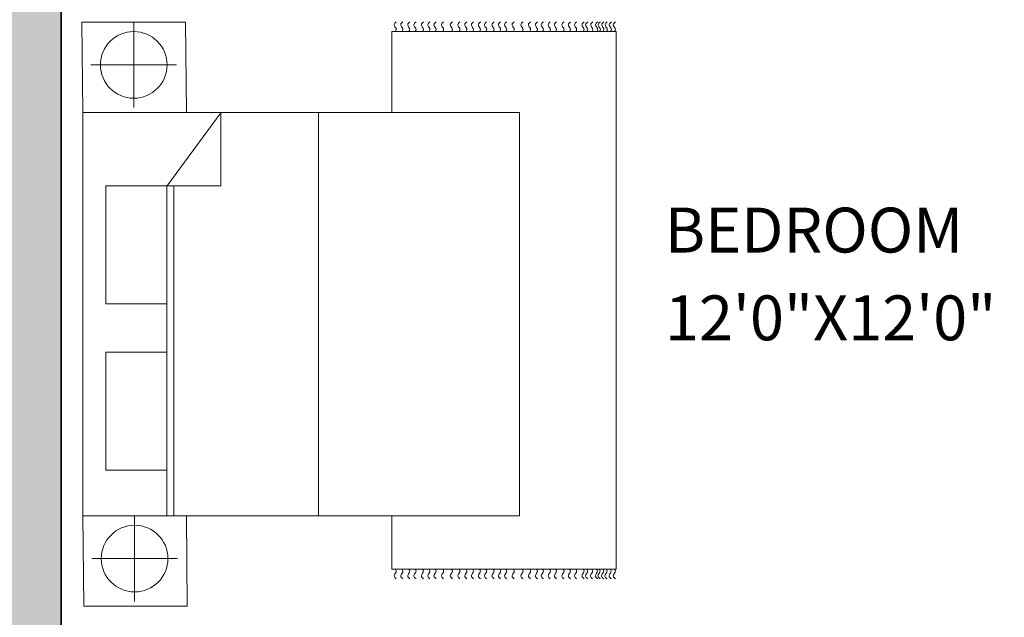
# Model space of a CAD drawing. Units: inches. Extents: x 1319 to 2030, y 219 to 1069.
# Tile 20 of 28: x 1433 to 1565, y 583 to 663. Entities that reach past the tile are written whole.
import ezdxf

# ---------------------------------------------------------------- set-up
doc = ezdxf.new("R2010")
doc.units = ezdxf.units.IN
doc.header["$MEASUREMENT"] = 0
for name, color, linetype, lineweight in [('A-AREA-IDEN', 250, 'Continuous', 18), ('A-WALL-PATT', 252, 'Continuous', 13), ('furniture', 250, 'Continuous', 18), ('walls', 250, 'Continuous', 35)]:
    doc.layers.add(name, color=color, linetype=linetype, lineweight=lineweight)
doc.styles.get("Standard").update_dxf_attribs({"font": 'arial.ttf'})

# ---------------------------------------------------------------- blocks, each defined once
blk = doc.blocks.new('CARPET')
at = {"layer": 'furniture'}
for p, q in [((-51.53, -98.11), (-51.53, -55.12)), ((-51.53, -55.12), (-41.27, -55.12)), ((36, -55.12), (51.55, -55.12)), ((51.55, -55.12), (51.55, -98.11)), ((51.55, -98.11), (-51.53, -98.11))]:
    blk.add_line(p, q, dxfattribs=at)
for points, knots in [([(-53.37, -55.99), (-53.22, -55.8), (-52.9, -55.41), (-52.34, -55.8), (-51.89, -56.08), (-51.65, -55.91), (-51.53, -55.83)], [0, 0, 0, 0, 0.653278, 1.290138, 1.740457, 2.114451, 2.114451, 2.114451, 2.114451]), ([(53.37, -55.99), (53.22, -55.8), (52.9, -55.41), (52.34, -55.8), (51.89, -56.08), (51.65, -55.91), (51.53, -55.83)], [0, 0, 0, 0, 0.653278, 1.290138, 1.740457, 2.114451, 2.114451, 2.114451, 2.114451]), ([(-53.37, -57.26), (-53.22, -57.07), (-52.9, -56.67), (-52.34, -57.07), (-51.89, -57.35), (-51.65, -57.17), (-51.53, -57.1)], [0, 0, 0, 0, 0.653278, 1.290138, 1.740457, 2.114451, 2.114451, 2.114451, 2.114451]), ([(-53.37, -58.59), (-53.22, -58.4), (-52.9, -58.01), (-52.34, -58.4), (-51.89, -58.68), (-51.65, -58.5), (-51.53, -58.43)], [0, 0, 0, 0, 0.653278, 1.290138, 1.740457, 2.114451, 2.114451, 2.114451, 2.114451]), ([(53.37, -57.26), (53.22, -57.07), (52.9, -56.67), (52.34, -57.07), (51.89, -57.35), (51.65, -57.17), (51.53, -57.1)], [0, 0, 0, 0, 0.653278, 1.290138, 1.740457, 2.114451, 2.114451, 2.114451, 2.114451]), ([(53.37, -58.59), (53.22, -58.4), (52.9, -58.01), (52.34, -58.4), (51.89, -58.68), (51.65, -58.5), (51.53, -58.43)], [0, 0, 0, 0, 0.653278, 1.290138, 1.740457, 2.114451, 2.114451, 2.114451, 2.114451]), ([(-53.37, -59.78), (-53.22, -59.58), (-52.9, -59.19), (-52.34, -59.58), (-51.89, -59.86), (-51.65, -59.69), (-51.53, -59.61)], [0, 0, 0, 0, 0.653278, 1.290138, 1.740457, 2.114451, 2.114451, 2.114451, 2.114451]), ([(53.37, -59.78), (53.22, -59.58), (52.9, -59.19), (52.34, -59.58), (51.89, -59.86), (51.65, -59.69), (51.53, -59.61)], [0, 0, 0, 0, 0.653278, 1.290138, 1.740457, 2.114451, 2.114451, 2.114451, 2.114451]), ([(-53.37, -61.22), (-53.22, -61.02), (-52.9, -60.63), (-52.34, -61.02), (-51.89, -61.3), (-51.65, -61.13), (-51.53, -61.05)], [0, 0, 0, 0, 0.653278, 1.290138, 1.740457, 2.114451, 2.114451, 2.114451, 2.114451]), ([(-53.37, -62.44), (-53.22, -62.25), (-52.9, -61.86), (-52.34, -62.25), (-51.89, -62.53), (-51.65, -62.36), (-51.53, -62.28)], [0, 0, 0, 0, 0.653278, 1.290138, 1.740457, 2.114451, 2.114451, 2.114451, 2.114451]), ([(53.37, -61.22), (53.22, -61.02), (52.9, -60.63), (52.34, -61.02), (51.89, -61.3), (51.65, -61.13), (51.53, -61.05)], [0, 0, 0, 0, 0.653278, 1.290138, 1.740457, 2.114451, 2.114451, 2.114451, 2.114451]), ([(53.37, -62.44), (53.22, -62.25), (52.9, -61.86), (52.34, -62.25), (51.89, -62.53), (51.65, -62.36), (51.53, -62.28)], [0, 0, 0, 0, 0.653278, 1.290138, 1.740457, 2.114451, 2.114451, 2.114451, 2.114451]), ([(-53.37, -63.63), (-53.22, -63.43), (-52.9, -63.04), (-52.34, -63.43), (-51.89, -63.72), (-51.65, -63.54), (-51.53, -63.46)], [0, 0, 0, 0, 0.653278, 1.290138, 1.740457, 2.114451, 2.114451, 2.114451, 2.114451]), ([(53.37, -63.63), (53.22, -63.43), (52.9, -63.04), (52.34, -63.43), (51.89, -63.72), (51.65, -63.54), (51.53, -63.46)], [0, 0, 0, 0, 0.653278, 1.290138, 1.740457, 2.114451, 2.114451, 2.114451, 2.114451]), ([(-53.37, -65.07), (-53.22, -64.87), (-52.9, -64.48), (-52.34, -64.87), (-51.89, -65.15), (-51.65, -64.98), (-51.53, -64.9)], [0, 0, 0, 0, 0.653278, 1.290138, 1.740457, 2.114451, 2.114451, 2.114451, 2.114451]), ([(53.37, -65.07), (53.22, -64.87), (52.9, -64.48), (52.34, -64.87), (51.89, -65.15), (51.65, -64.98), (51.53, -64.9)], [0, 0, 0, 0, 0.653278, 1.290138, 1.740457, 2.114451, 2.114451, 2.114451, 2.114451]), ([(-53.37, -66.76), (-53.22, -66.56), (-52.9, -66.17), (-52.34, -66.56), (-51.89, -66.84), (-51.65, -66.67), (-51.53, -66.59)], [0, 0, 0, 0, 0.653278, 1.290138, 1.740457, 2.114451, 2.114451, 2.114451, 2.114451]), ([(-53.37, -68.2), (-53.22, -68), (-52.9, -67.61), (-52.34, -68), (-51.89, -68.28), (-51.65, -68.11), (-51.53, -68.03)], [0, 0, 0, 0, 0.653278, 1.290138, 1.740457, 2.114451, 2.114451, 2.114451, 2.114451]), ([(53.37, -66.76), (53.22, -66.56), (52.9, -66.17), (52.34, -66.56), (51.89, -66.84), (51.65, -66.67), (51.53, -66.59)], [0, 0, 0, 0, 0.653278, 1.290138, 1.740457, 2.114451, 2.114451, 2.114451, 2.114451]), ([(53.37, -68.2), (53.22, -68), (52.9, -67.61), (52.34, -68), (51.89, -68.28), (51.65, -68.11), (51.53, -68.03)], [0, 0, 0, 0, 0.653278, 1.290138, 1.740457, 2.114451, 2.114451, 2.114451, 2.114451]), ([(-53.37, -69.53), (-53.22, -69.33), (-52.9, -68.94), (-52.34, -69.33), (-51.89, -69.61), (-51.65, -69.44), (-51.53, -69.36)], [0, 0, 0, 0, 0.653278, 1.290138, 1.740457, 2.114451, 2.114451, 2.114451, 2.114451]), ([(53.37, -69.53), (53.22, -69.33), (52.9, -68.94), (52.34, -69.33), (51.89, -69.61), (51.65, -69.44), (51.53, -69.36)], [0, 0, 0, 0, 0.653278, 1.290138, 1.740457, 2.114451, 2.114451, 2.114451, 2.114451]), ([(-53.37, -70.79), (-53.22, -70.6), (-52.9, -70.21), (-52.34, -70.6), (-51.89, -70.88), (-51.65, -70.7), (-51.53, -70.63)], [0, 0, 0, 0, 0.653278, 1.290138, 1.740457, 2.114451, 2.114451, 2.114451, 2.114451]), ([(-53.37, -72.12), (-53.22, -71.93), (-52.9, -71.54), (-52.34, -71.93), (-51.89, -72.21), (-51.65, -72.04), (-51.53, -71.96)], [0, 0, 0, 0, 0.653278, 1.290138, 1.740457, 2.114451, 2.114451, 2.114451, 2.114451]), ([(53.37, -70.79), (53.22, -70.6), (52.9, -70.21), (52.34, -70.6), (51.89, -70.88), (51.65, -70.7), (51.53, -70.63)], [0, 0, 0, 0, 0.653278, 1.290138, 1.740457, 2.114451, 2.114451, 2.114451, 2.114451]), ([(53.37, -72.12), (53.22, -71.93), (52.9, -71.54), (52.34, -71.93), (51.89, -72.21), (51.65, -72.04), (51.53, -71.96)], [0, 0, 0, 0, 0.653278, 1.290138, 1.740457, 2.114451, 2.114451, 2.114451, 2.114451]), ([(-53.37, -73.31), (-53.22, -73.11), (-52.9, -72.72), (-52.34, -73.11), (-51.89, -73.4), (-51.65, -73.22), (-51.53, -73.14)], [0, 0, 0, 0, 0.653278, 1.290138, 1.740457, 2.114451, 2.114451, 2.114451, 2.114451]), ([(53.37, -73.31), (53.22, -73.11), (52.9, -72.72), (52.34, -73.11), (51.89, -73.4), (51.65, -73.22), (51.53, -73.14)], [0, 0, 0, 0, 0.653278, 1.290138, 1.740457, 2.114451, 2.114451, 2.114451, 2.114451]), ([(-53.37, -74.75), (-53.22, -74.55), (-52.9, -74.16), (-52.34, -74.55), (-51.89, -74.83), (-51.65, -74.66), (-51.53, -74.58)], [0, 0, 0, 0, 0.653278, 1.290138, 1.740457, 2.114451, 2.114451, 2.114451, 2.114451]), ([(53.37, -74.75), (53.22, -74.55), (52.9, -74.16), (52.34, -74.55), (51.89, -74.83), (51.65, -74.66), (51.53, -74.58)], [0, 0, 0, 0, 0.653278, 1.290138, 1.740457, 2.114451, 2.114451, 2.114451, 2.114451]), ([(-53.37, -75.98), (-53.22, -75.78), (-52.9, -75.39), (-52.34, -75.78), (-51.89, -76.06), (-51.65, -75.89), (-51.53, -75.81)], [0, 0, 0, 0, 0.653278, 1.290138, 1.740457, 2.114451, 2.114451, 2.114451, 2.114451]), ([(-53.37, -77.16), (-53.22, -76.96), (-52.9, -76.57), (-52.34, -76.96), (-51.89, -77.25), (-51.65, -77.07), (-51.53, -76.99)], [0, 0, 0, 0, 0.653278, 1.290138, 1.740457, 2.114451, 2.114451, 2.114451, 2.114451]), ([(53.37, -75.98), (53.22, -75.78), (52.9, -75.39), (52.34, -75.78), (51.89, -76.06), (51.65, -75.89), (51.53, -75.81)], [0, 0, 0, 0, 0.653278, 1.290138, 1.740457, 2.114451, 2.114451, 2.114451, 2.114451]), ([(53.37, -77.16), (53.22, -76.96), (52.9, -76.57), (52.34, -76.96), (51.89, -77.25), (51.65, -77.07), (51.53, -76.99)], [0, 0, 0, 0, 0.653278, 1.290138, 1.740457, 2.114451, 2.114451, 2.114451, 2.114451]), ([(-53.37, -78.6), (-53.22, -78.4), (-52.9, -78.01), (-52.34, -78.4), (-51.89, -78.68), (-51.65, -78.51), (-51.53, -78.43)], [0, 0, 0, 0, 0.653278, 1.290138, 1.740457, 2.114451, 2.114451, 2.114451, 2.114451]), ([(53.37, -78.6), (53.22, -78.4), (52.9, -78.01), (52.34, -78.4), (51.89, -78.68), (51.65, -78.51), (51.53, -78.43)], [0, 0, 0, 0, 0.653278, 1.290138, 1.740457, 2.114451, 2.114451, 2.114451, 2.114451]), ([(-53.37, -80.29), (-53.22, -80.09), (-52.9, -79.7), (-52.34, -80.09), (-51.89, -80.37), (-51.65, -80.2), (-51.53, -80.12)], [0, 0, 0, 0, 0.653278, 1.290138, 1.740457, 2.114451, 2.114451, 2.114451, 2.114451]), ([(53.37, -80.29), (53.22, -80.09), (52.9, -79.7), (52.34, -80.09), (51.89, -80.37), (51.65, -80.2), (51.53, -80.12)], [0, 0, 0, 0, 0.653278, 1.290138, 1.740457, 2.114451, 2.114451, 2.114451, 2.114451]), ([(-53.37, -81.73), (-53.22, -81.53), (-52.9, -81.14), (-52.34, -81.53), (-51.89, -81.81), (-51.65, -81.64), (-51.53, -81.56)], [0, 0, 0, 0, 0.653278, 1.290138, 1.740457, 2.114451, 2.114451, 2.114451, 2.114451]), ([(-53.37, -83.06), (-53.22, -82.86), (-52.9, -82.47), (-52.34, -82.86), (-51.89, -83.14), (-51.65, -82.97), (-51.53, -82.89)], [0, 0, 0, 0, 0.653278, 1.290138, 1.740457, 2.114451, 2.114451, 2.114451, 2.114451]), ([(53.37, -81.73), (53.22, -81.53), (52.9, -81.14), (52.34, -81.53), (51.89, -81.81), (51.65, -81.64), (51.53, -81.56)], [0, 0, 0, 0, 0.653278, 1.290138, 1.740457, 2.114451, 2.114451, 2.114451, 2.114451]), ([(53.37, -83.06), (53.22, -82.86), (52.9, -82.47), (52.34, -82.86), (51.89, -83.14), (51.65, -82.97), (51.53, -82.89)], [0, 0, 0, 0, 0.653278, 1.290138, 1.740457, 2.114451, 2.114451, 2.114451, 2.114451]), ([(-53.37, -84.18), (-53.22, -83.99), (-52.9, -83.6), (-52.34, -83.99), (-51.89, -84.27), (-51.65, -84.09), (-51.53, -84.02)], [0, 0, 0, 0, 0.653278, 1.290138, 1.740457, 2.114451, 2.114451, 2.114451, 2.114451]), ([(53.37, -84.18), (53.22, -83.99), (52.9, -83.6), (52.34, -83.99), (51.89, -84.27), (51.65, -84.09), (51.53, -84.02)], [0, 0, 0, 0, 0.653278, 1.290138, 1.740457, 2.114451, 2.114451, 2.114451, 2.114451]), ([(-53.37, -85.51), (-53.22, -85.32), (-52.9, -84.93), (-52.34, -85.32), (-51.89, -85.6), (-51.65, -85.42), (-51.53, -85.35)], [0, 0, 0, 0, 0.653278, 1.290138, 1.740457, 2.114451, 2.114451, 2.114451, 2.114451]), ([(-53.37, -86.7), (-53.22, -86.5), (-52.9, -86.11), (-52.34, -86.5), (-51.89, -86.78), (-51.65, -86.61), (-51.53, -86.53)], [0, 0, 0, 0, 0.653278, 1.290138, 1.740457, 2.114451, 2.114451, 2.114451, 2.114451]), ([(53.37, -85.51), (53.22, -85.32), (52.9, -84.93), (52.34, -85.32), (51.89, -85.6), (51.65, -85.42), (51.53, -85.35)], [0, 0, 0, 0, 0.653278, 1.290138, 1.740457, 2.114451, 2.114451, 2.114451, 2.114451]), ([(53.37, -86.7), (53.22, -86.5), (52.9, -86.11), (52.34, -86.5), (51.89, -86.78), (51.65, -86.61), (51.53, -86.53)], [0, 0, 0, 0, 0.653278, 1.290138, 1.740457, 2.114451, 2.114451, 2.114451, 2.114451]), ([(-53.37, -88.14), (-53.22, -87.94), (-52.9, -87.55), (-52.34, -87.94), (-51.89, -88.22), (-51.65, -88.05), (-51.53, -87.97)], [0, 0, 0, 0, 0.653278, 1.290138, 1.740457, 2.114451, 2.114451, 2.114451, 2.114451]), ([(53.37, -88.14), (53.22, -87.94), (52.9, -87.55), (52.34, -87.94), (51.89, -88.22), (51.65, -88.05), (51.53, -87.97)], [0, 0, 0, 0, 0.653278, 1.290138, 1.740457, 2.114451, 2.114451, 2.114451, 2.114451]), ([(-53.37, -89.36), (-53.22, -89.17), (-52.9, -88.78), (-52.34, -89.17), (-51.89, -89.45), (-51.65, -89.28), (-51.53, -89.2)], [0, 0, 0, 0, 0.653278, 1.290138, 1.740457, 2.114451, 2.114451, 2.114451, 2.114451]), ([(-53.37, -90.55), (-53.22, -90.35), (-52.9, -89.96), (-52.34, -90.35), (-51.89, -90.64), (-51.65, -90.46), (-51.53, -90.38)], [0, 0, 0, 0, 0.653278, 1.290138, 1.740457, 2.114451, 2.114451, 2.114451, 2.114451]), ([(53.37, -89.36), (53.22, -89.17), (52.9, -88.78), (52.34, -89.17), (51.89, -89.45), (51.65, -89.28), (51.53, -89.2)], [0, 0, 0, 0, 0.653278, 1.290138, 1.740457, 2.114451, 2.114451, 2.114451, 2.114451]), ([(53.37, -90.55), (53.22, -90.35), (52.9, -89.96), (52.34, -90.35), (51.9, -90.63), (51.66, -90.47), (51.55, -90.4)], [0, 0, 0, 0, 0.653278, 1.290138, 1.740457, 2.0926, 2.0926, 2.0926, 2.0926]), ([(-53.37, -91.99), (-53.22, -91.79), (-52.9, -91.4), (-52.34, -91.79), (-51.89, -92.07), (-51.65, -91.9), (-51.53, -91.82)], [0, 0, 0, 0, 0.653278, 1.290138, 1.740457, 2.114451, 2.114451, 2.114451, 2.114451]), ([(-53.37, -92.69), (-53.22, -92.48), (-52.9, -92.08), (-52.35, -92.49), (-51.89, -92.77), (-51.65, -92.6), (-51.53, -92.52)], [0, 0, 0, 0, 0.663904, 1.307406, 1.757725, 2.131719, 2.131719, 2.131719, 2.131719]), ([(53.37, -91.99), (53.22, -91.79), (52.9, -91.4), (52.34, -91.79), (51.9, -92.07), (51.66, -91.91), (51.55, -91.83)], [0, 0, 0, 0, 0.653278, 1.290138, 1.740457, 2.0926, 2.0926, 2.0926, 2.0926]), ([(53.37, -92.69), (53.22, -92.49), (52.9, -92.09), (52.34, -92.49), (51.9, -92.77), (51.66, -92.61), (51.55, -92.53)], [0, 0, 0, 0, 0.656792, 1.295826, 1.746145, 2.098292, 2.098292, 2.098292, 2.098292]), ([(-53.37, -93.61), (-53.22, -93.42), (-52.9, -93.03), (-52.34, -93.42), (-51.89, -93.7), (-51.65, -93.52), (-51.53, -93.45)], [0, 0, 0, 0, 0.653278, 1.290138, 1.740457, 2.114451, 2.114451, 2.114451, 2.114451]), ([(-53.37, -94.55), (-53.22, -94.35), (-52.9, -93.96), (-52.34, -94.35), (-51.89, -94.63), (-51.65, -94.46), (-51.53, -94.38)], [0, 0, 0, 0, 0.653278, 1.290138, 1.740457, 2.114451, 2.114451, 2.114451, 2.114451]), ([(53.37, -93.66), (53.22, -93.46), (52.9, -93.07), (52.34, -93.46), (51.9, -93.74), (51.66, -93.58), (51.55, -93.5)], [0, 0, 0, 0, 0.653278, 1.290138, 1.740457, 2.0926, 2.0926, 2.0926, 2.0926]), ([(53.37, -94.59), (53.22, -94.4), (52.9, -94.01), (52.34, -94.4), (51.9, -94.68), (51.66, -94.51), (51.55, -94.44)], [0, 0, 0, 0, 0.653278, 1.290138, 1.740457, 2.0926, 2.0926, 2.0926, 2.0926]), ([(-53.37, -95.05), (-53.22, -94.85), (-52.9, -94.46), (-52.34, -94.85), (-51.89, -95.14), (-51.65, -94.96), (-51.53, -94.88)], [0, 0, 0, 0, 0.653278, 1.290138, 1.740457, 2.114451, 2.114451, 2.114451, 2.114451]), ([(-53.37, -95.73), (-53.22, -95.54), (-52.9, -95.15), (-52.34, -95.54), (-51.89, -95.82), (-51.65, -95.65), (-51.53, -95.57)], [0, 0, 0, 0, 0.653278, 1.290138, 1.740457, 2.114451, 2.114451, 2.114451, 2.114451]), ([(-53.37, -96.38), (-53.22, -96.18), (-52.9, -95.79), (-52.34, -96.18), (-51.89, -96.47), (-51.65, -96.29), (-51.53, -96.21)], [0, 0, 0, 0, 0.653278, 1.290138, 1.740457, 2.114451, 2.114451, 2.114451, 2.114451]), ([(53.37, -95.78), (53.22, -95.58), (52.9, -95.19), (52.34, -95.58), (51.89, -95.86), (51.65, -95.69), (51.53, -95.61)], [0, 0, 0, 0, 0.653278, 1.290138, 1.740457, 2.114451, 2.114451, 2.114451, 2.114451]), ([(53.37, -96.43), (53.22, -96.23), (52.9, -95.84), (52.34, -96.23), (51.89, -96.51), (51.65, -96.34), (51.53, -96.26)], [0, 0, 0, 0, 0.653278, 1.290138, 1.740457, 2.114451, 2.114451, 2.114451, 2.114451]), ([(53.37, -95.1), (53.22, -94.9), (52.9, -94.51), (52.34, -94.9), (51.9, -95.18), (51.66, -95.02), (51.55, -94.94)], [0, 0, 0, 0, 0.653278, 1.290138, 1.740457, 2.0926, 2.0926, 2.0926, 2.0926]), ([(-53.37, -97.17), (-53.22, -96.98), (-52.9, -96.59), (-52.34, -96.98), (-51.89, -97.26), (-51.65, -97.08), (-51.53, -97.01)], [0, 0, 0, 0, 0.653278, 1.290138, 1.740457, 2.114451, 2.114451, 2.114451, 2.114451]), ([(-53.37, -97.99), (-53.22, -97.79), (-52.9, -97.4), (-52.34, -97.79), (-51.89, -98.08), (-51.65, -97.9), (-51.53, -97.82)], [0, 0, 0, 0, 0.653278, 1.290138, 1.740457, 2.114451, 2.114451, 2.114451, 2.114451]), ([(53.37, -97.22), (53.22, -97.02), (52.9, -96.63), (52.34, -97.02), (51.89, -97.3), (51.65, -97.13), (51.53, -97.05)], [0, 0, 0, 0, 0.653278, 1.290138, 1.740457, 2.114451, 2.114451, 2.114451, 2.114451]), ([(53.37, -97.99), (53.22, -97.79), (52.9, -97.4), (52.34, -97.79), (51.89, -98.08), (51.65, -97.9), (51.53, -97.82)], [0, 0, 0, 0, 0.653278, 1.290138, 1.740457, 2.114451, 2.114451, 2.114451, 2.114451])]:
    blk.add_open_spline(points, degree=3, knots=knots, dxfattribs=at)
blk = doc.blocks.new('A$C58D270C6')
at = {"layer": 'furniture'}
for p, q in [((9.09, 124.13), (9.09, 108.87)), ((1.46, 116.5), (16.73, 116.5)), ((14.97, 94.84), (24.62, 107.92)), ((24.62, 94.93), (24.62, 107.92)), ((42.08, 108), (42.08, 36)), ((14.97, 94.93), (24.62, 94.93)), ((16.22, 94.93), (16.22, 36)), ((14.97, 94.84), (14.97, 36)), ((9.25, 36), (9.25, 20.74)), ((1.62, 28.37), (16.88, 28.37))]:
    blk.add_line(p, q, dxfattribs=at)
for points in [[(18.5, 108), (18.34, 124.13), (-0.16, 124.13), (0, 108)], [(0, 108), (77.91, 108), (77.91, 36), (0, 36)], [(4.09, 94.93), (14.97, 94.93), (14.97, 73.83), (4.09, 73.83)], [(4.09, 65.23), (14.97, 65.23), (14.97, 44.13), (4.09, 44.13)], [(18.65, 19.87), (18.5, 36), (0, 36), (0.16, 19.87)]]:
    blk.add_lwpolyline(points, close=True, dxfattribs=at)
for centre in [(9.09, 116.5), (9.25, 28.37)]:
    blk.add_circle(centre, 5.95, dxfattribs=at)
at = {"layer": 'furniture', "xscale": 0.9312884925094044, "yscale": 0.9312884925094044, "zscale": 0.9312884925094044, "rotation": 90}
blk.add_blockref('CARPET', (3.79, 74.47), dxfattribs=at)

msp = doc.modelspace()

# ---------------------------------------------------------------- hatches: boundary and pattern name
at = {"layer": 'A-WALL-PATT'}
h = msp.add_hatch(color=256, dxfattribs=at)
h.dxf.hatch_style = 1
h.paths.add_polyline_path([(1856.292, 860.616), (1812.343, 860.616), (1812.343, 851.616), (1812.343, 700.993), (1816.843, 700.993), (1816.843, 851.616), (1856.292, 851.616)])
h.paths.add_polyline_path([(1960.843, 663.616), (1812.343, 663.616), (1782.783, 663.616), (1782.783, 659.116), (1812.343, 659.116), (1960.843, 659.116)])
h.paths.add_polyline_path([(1857.424, 659.116), (1852.924, 659.116), (1852.924, 616.807), (1857.424, 616.807)])
h.paths.add_polyline_path([(1735.843, 661.727), (1731.843, 661.727), (1636.133, 661.727), (1636.133, 657.227), (1731.343, 657.227), (1731.343, 481.227), (1618.616, 481.227), (1618.616, 472.227), (1639.343, 472.227), (1639.343, 384.227), (1627.044, 384.227), (1627.044, 375.227), (1648.343, 375.227), (1648.343, 384.227), (1648.343, 472.227), (1750.706, 472.227), (1750.706, 481.227), (1735.843, 481.227), (1735.843, 657.727)])
h.paths.add_polyline_path([(1587.343, 481.227), (1578.343, 481.227), (1578.343, 375.227), (1597.622, 375.227), (1597.622, 384.227), (1587.343, 384.227)])
h.paths.add_polyline_path([(1769.593, 384.227), (1693.482, 384.227), (1693.482, 375.227), (1769.593, 375.227)])
h.paths.add_polyline_path([(1775.828, 481.227), (1765.831, 481.227), (1765.831, 472.227), (1775.828, 472.227)])
h.paths.add_polyline_path([(1824.625, 481.227), (1820.343, 481.227), (1820.343, 476.727), (1824.625, 476.727), (1824.625, 477.545)], flags=0)
h.paths.add_polyline_path([(1896.843, 481.227), (1852.26, 481.227), (1852.26, 476.727), (1892.343, 476.727), (1892.343, 384.227), (1881.742, 384.227), (1881.742, 375.227), (1913.435, 375.227), (1913.435, 384.227), (1896.843, 384.227)])
h.paths.add_polyline_path([(1960.843, 481.227), (1931.341, 481.227), (1931.341, 476.727), (1960.843, 476.727)])
h.paths.add_polyline_path([(1736.343, 918.227), (1731.843, 918.227), (1731.843, 890.227), (1582.843, 890.227), (1582.843, 781.727), (1582.843, 769.171), (1587.343, 769.171), (1587.343, 781.727), (1587.343, 885.727), (1731.843, 885.727), (1731.843, 851.616), (1736.343, 851.616), (1736.343, 890.227)])
h.paths.add_polyline_path([(1781.022, 860.616), (1773.021, 860.616, -0.0322281), (1773.289, 856.464), (1773.289, 851.616), (1781.022, 851.616)])
h.paths.add_polyline_path([(1587.343, 946.227), (1582.843, 946.227), (1582.843, 926.136), (1587.343, 926.136)])
h.paths.add_polyline_path([(1647.843, 946.227), (1643.343, 946.227), (1643.343, 926.136), (1647.843, 926.136)])
h.paths.add_polyline_path([(1543.343, 786.227), (1429.843, 786.227), (1429.843, 757.555), (1434.343, 757.555), (1438.843, 757.555), (1438.843, 781.727), (1543.343, 781.727)])
h.paths.add_polyline_path([(1543.343, 781.727), (1538.843, 781.727), (1538.843, 709.727), (1534.597, 709.727), (1534.597, 705.227), (1543.343, 705.227), (1543.343, 709.727)])
h.paths.add_polyline_path([(1499.955, 709.727), (1438.843, 709.727), (1438.843, 734.463), (1429.843, 734.463), (1429.843, 552.227), (1470.241, 552.227), (1470.241, 561.227), (1438.843, 561.227), (1438.843, 705.227), (1499.955, 705.227)])
h.paths.add_polyline_path([(1587.343, 709.727), (1582.843, 709.727), (1582.843, 561.227), (1543.433, 561.227), (1543.433, 552.227), (1587.343, 552.227)])
h.paths.add_polyline_path([(1546.835, 709.727), (1543.343, 709.727), (1543.343, 705.227), (1546.835, 705.227)])
h.paths.add_polyline_path([(1582.843, 709.727), (1579.15, 709.727), (1579.15, 705.227), (1582.843, 705.227)], flags=17)
h.paths.add_polyline_path([(1548.368, 786.227), (1543.343, 786.227), (1543.343, 781.727), (1548.368, 781.727)])
h.paths.add_polyline_path([(1582.843, 786.227), (1580.683, 786.227), (1580.683, 781.727), (1582.843, 781.727)])
h.paths.add_polyline_path([(1587.343, 892.402), (1582.843, 892.402), (1582.843, 890.227), (1587.343, 890.227)], flags=17)
h.paths.add_polyline_path([(1647.843, 892.402), (1643.343, 892.402), (1643.343, 890.227), (1647.843, 890.227)], flags=17)
h.paths.add_polyline_path([(1740.974, 856.464), (1740.974, 860.616), (1736.343, 860.616), (1736.343, 851.616), (1740.974, 851.616)])
h.paths.add_polyline_path([(1853.989, 384.227), (1820.343, 384.227), (1820.343, 402.924), (1815.843, 402.924), (1815.843, 375.227), (1853.989, 375.227)])
h.paths.add_polyline_path([(1892.343, 436.227), (1820.343, 436.227), (1820.343, 481.227), (1815.843, 481.227), (1815.843, 431.727), (1892.343, 431.727)])
h.paths.add_polyline_path([(1849.175, 481.227), (1824.625, 481.227), (1824.625, 477.545), (1825.699, 477.545), (1825.699, 453.018, 0.4014527), (1849.175, 477.545)], flags=0)
h.paths.add_polyline_path([(1960.843, 384.227), (1941.188, 384.227), (1941.188, 375.227), (1960.843, 375.227)])
h.paths.add_polyline_path([(1902.267, 481.227), (1896.843, 481.227), (1896.843, 476.727), (1902.267, 476.727), (1902.267, 477.44)], flags=0)

# ---------------------------------------------------------------- linework, layer by layer
at = {"layer": 'walls'}
msp.add_line((1438.843, 561.227), (1438.843, 705.227), dxfattribs=at)

# ---------------------------------------------------------------- block references
at = {"layer": 'furniture', "xscale": 0.7500000390647866, "yscale": 0.7500000390647866, "zscale": 0.7500000390647866}
msp.add_blockref('A$C58D270C6', (1441.723, 569.9), dxfattribs=at)

# ---------------------------------------------------------------- texts
at = {"layer": 'A-AREA-IDEN'}
for s, height, p in [('BEDROOM', 6.0112, (1519.625, 632.15)), ('12\'0"X12\'0"', 6.01124, (1519.625, 620.401))]:
    msp.add_text(s, height=height, dxfattribs=at).set_placement(p)

doc.saveas('drawing.dxf')
